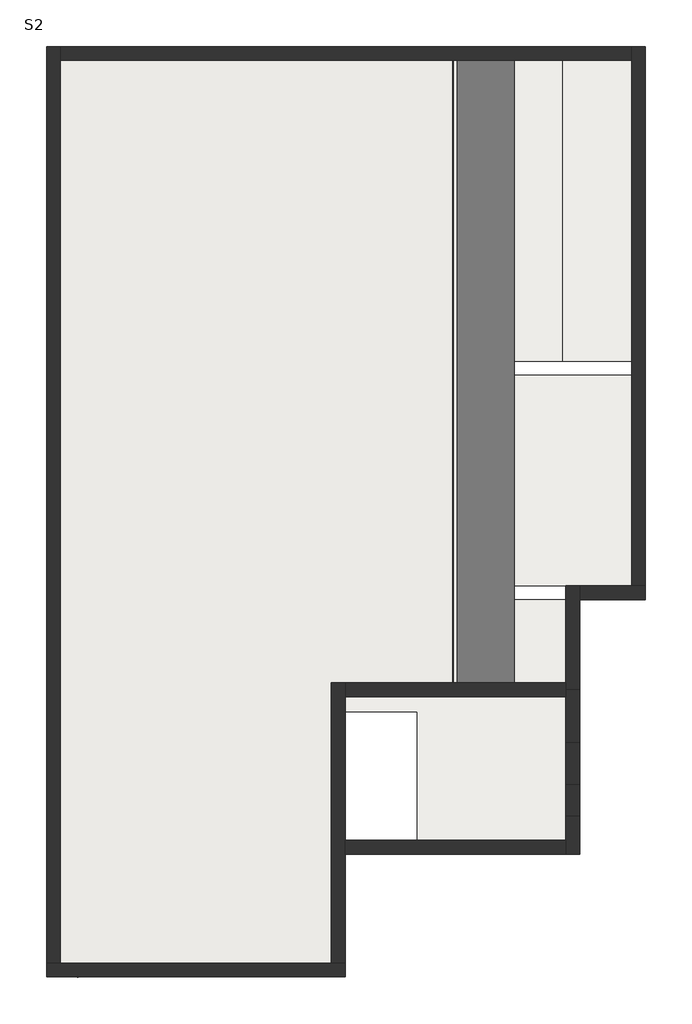
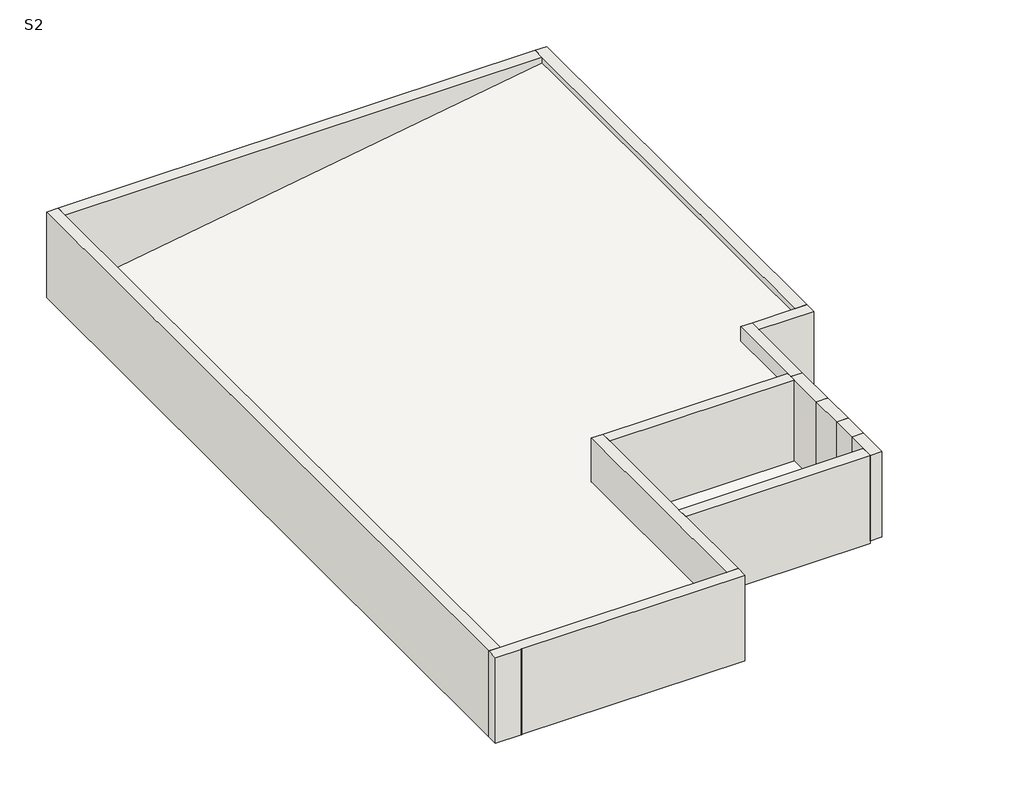
# One storey: 13 walls, 9 coverings, 2 roofs, 1 proxy.
"""IFC4 building model written with IfcOpenShell, lengths in millimetres."""

from ifc_helpers import new_model, si_unit, point, frame, frame_2d, origin, place, context, project, spatial, polyline, circle_curve, trimmed, segment, composite_curve, outline, extrude, faceted_brep, element, save
from ifc_brep_helpers import plane_surface, revolved_surface, advanced_brep

model = new_model("IFC4")

# Units and contexts
model_context = context("Model", 3, world=origin())
ifc_project = project(units=[si_unit("LENGTHUNIT", "METRE", prefix="MILLI")], contexts=[model_context])

# Site, building, storey
site = spatial("IfcSite", under=ifc_project)
building = spatial("IfcBuilding", under=site)
storey = spatial("IfcBuildingStorey", under=building, Name="S2", Elevation=7200.0)

# Proxy
placement = place(None, origin())
element("IfcBuildingElementProxy", 1, Name="Reveal", ObjectType="Reveal", at=placement, inside=storey, context=model_context, shape_type="SweptSolid", body=[
    extrude(outline(composite_curve([segment(trimmed(circle_curve(frame_2d((-9788.8712297, -10317.0014262)), 7.5), [point((-9788.8712297, -10324.5014262))], [point((-9788.8712297, -10309.5014262))], False, "CARTESIAN"), True, "CONTINUOUS"), segment(trimmed(circle_curve(frame_2d((-9788.8712297, -10317.0014262)), 7.5), [point((-9788.8712297, -10309.5014262))], [point((-9788.8712297, -10324.5014262))], False, "CARTESIAN"), True, "CONTINUOUS")], self_intersect=False)), frame((0.0, 0.0, 7200.0), z_axis=(0.0, 0.0, 1.0), x_axis=(1.0, 0.0, 0.0)), (0.0, 0.0, 1.0), 1800.0),
])

# Coverings
element("IfcCovering", 2, ObjectType="600 x 1200mm grid", at=placement, inside=storey, context=model_context, shape_type="Brep", body=[
    faceted_brep([(-8268.1448516, -9277.0014262, 6953.3191854), (-9078.1448516, -10087.0014262, 7253.3191854), (-5941.5057893, -10087.0014262, 7253.3191854), (-6751.5057893, -9277.0014262, 6953.3191854), (-8268.1448516, -9277.0014262, 6900.0), (-6751.5057893, -9277.0014262, 6900.0), (-5941.5057893, -10087.0014262, 7200.0), (-9078.1448516, -10087.0014262, 7200.0)], [[[0, 1, 2, 3]], [[4, 5, 6, 7]], [[1, 0, 4, 7]], [[2, 1, 7, 6]], [[3, 2, 6, 5]], [[0, 3, 5, 4]]]),
])
element("IfcCovering", 3, ObjectType="600 x 1200mm grid", at=placement, inside=storey, context=model_context, shape_type="SweptSolid", body=[
    extrude(outline(polyline([(-5578.8712297, -2725.4326238), (-7378.8712297, -2725.4326238), (-7378.8712297, -2955.4326238), (-5578.8712297, -2955.4326238), (-5578.8712297, -10124.3668665), (-6656.23667, -9047.0014262), (-8363.4139709, -9047.0014262), (-9403.4139709, -10087.0014262), (-10078.8712297, -10087.0014262), (-10078.8712297, -2955.4326238), (-9478.8712297, -2955.4326238), (-9478.8712297, -2725.4326238), (-10078.8712297, -2725.4326238), (-10078.8712297, -317.0014262), (-5578.8712297, -317.0014262), (-5578.8712297, -2725.4326238)])), frame((0.0, 0.0, 7150.0), z_axis=(0.0, 0.0, 1.0), x_axis=(1.0, 0.0, 0.0)), (0.0, 0.0, 1.0), 50.0),
])
element("IfcCovering", 4, ObjectType="600 x 1200mm grid", at=placement, inside=storey, context=model_context, shape_type="SweptSolid", body=[
    extrude(outline(polyline([(-5348.8712297, -5662.0014262), (-1678.8712297, -5662.0014262), (-1678.8712297, -6422.0014262), (-1678.8712297, -7122.0014262), (-1678.8712297, -7637.0014262), (-1678.8712297, -8047.0014262), (-4148.8712297, -8047.0014262), (-4148.8712297, -5912.0014262), (-5348.8712297, -5912.0014262), (-5348.8712297, -5662.0014262)])), frame((0.0, 0.0, 7150.0), z_axis=(0.0, 0.0, 1.0), x_axis=(1.0, 0.0, 0.0)), (0.0, 0.0, 1.0), 50.0),
])
element("IfcCovering", 5, ObjectType="600 x 1200mm grid", at=placement, inside=storey, context=model_context, shape_type="SweptSolid", body=[
    extrude(outline(polyline([(-5348.8712297, -5432.0014262), (-5348.8712297, -4047.0014262), (-1678.8712297, -4047.0014262), (-1678.8712297, -5432.0014262), (-5348.8712297, -5432.0014262)])), frame((0.0, 0.0, 7150.0), z_axis=(0.0, 0.0, 1.0), x_axis=(1.0, 0.0, 0.0)), (0.0, 0.0, 1.0), 50.0),
])
element("IfcCovering", 6, ObjectType="600 x 1200mm grid", at=placement, inside=storey, context=model_context, shape_type="SweptSolid", body=[
    extrude(outline(polyline([(-5348.8712297, -317.0014262), (-588.8712297, -317.0014262), (-588.8712297, -3817.0014262), (-5348.8712297, -3817.0014262), (-5348.8712297, -317.0014262)])), frame((0.0, 0.0, 7150.0), z_axis=(0.0, 0.0, 1.0), x_axis=(1.0, 0.0, 0.0)), (0.0, 0.0, 1.0), 50.0),
])
element("IfcCovering", 7, ObjectType="600 x 1200mm grid", at=placement, inside=storey, context=model_context, shape_type="SweptSolid", body=[
    extrude(outline(polyline([(-10078.8712297, 4912.9985738), (-5348.8712297, 4912.9985738), (-5348.8712297, 1822.9985738), (-5118.8712297, 1822.9985738), (-5118.8712297, 4912.9985738), (-1741.8392368, 4912.9985738), (-1741.8392368, -87.0014262), (-5118.8712297, -87.0014262), (-5118.8712297, -502.0014262), (-5348.8712297, -502.0014262), (-5348.8712297, -87.0014262), (-10078.8712297, -87.0014262), (-10078.8712297, 4912.9985738)])), frame((0.0, 0.0, 7150.0), z_axis=(0.0, 0.0, 1.0), x_axis=(1.0, 0.0, 0.0)), (0.0, 0.0, 1.0), 50.0),
])
element("IfcCovering", 8, ObjectType="600 x 1200mm grid", at=placement, inside=storey, context=model_context, shape_type="SweptSolid", body=[
    extrude(outline(polyline([(-3590.0839081, 4912.9985738), (-588.8712297, 4912.9985738), (-588.8712297, -87.0014262), (-3590.0839081, -87.0014262), (-3590.0839081, 4912.9985738)])), frame((0.0, 0.0, 7150.0), z_axis=(0.0, 0.0, 1.0), x_axis=(1.0, 0.0, 0.0)), (0.0, 0.0, 1.0), 50.0),
])
element("IfcCovering", 9, ObjectType="600 x 1200mm grid", at=placement, inside=storey, context=model_context, shape_type="SweptSolid", body=[
    extrude(outline(polyline([(-5348.8712297, -5662.0014262), (-1678.8712297, -5662.0014262), (-1678.8712297, -6422.0014262), (-1678.8712297, -7122.0014262), (-1678.8712297, -7637.0014262), (-1678.8712297, -8047.0014262), (-4148.8712297, -8047.0014262), (-4148.8712297, -5912.0014262), (-5348.8712297, -5912.0014262), (-5348.8712297, -5662.0014262)])), frame((0.0, 0.0, 7200.0), z_axis=(0.0, 0.0, 1.0), x_axis=(1.0, 0.0, 0.0)), (0.0, 0.0, 1.0), 50.0),
])
element("IfcCovering", 10, ObjectType="600 x 1200mm grid", at=placement, inside=storey, context=model_context, shape_type="SweptSolid", body=[
    extrude(outline(polyline([(-5348.8712297, -5662.0014262), (-1678.8712297, -5662.0014262), (-1678.8712297, -6422.0014262), (-1678.8712297, -7122.0014262), (-1678.8712297, -7637.0014262), (-1678.8712297, -8047.0014262), (-4148.8712297, -8047.0014262), (-4148.8712297, -5912.0014262), (-5348.8712297, -5912.0014262), (-5348.8712297, -5662.0014262)])), frame((0.0, 0.0, 7250.0), z_axis=(0.0, 0.0, 1.0), x_axis=(1.0, 0.0, 0.0)), (0.0, 0.0, 1.0), 50.0),
])

# Roofs
element("IfcRoof", 11, ObjectType="150", at=placement, inside=storey, context=model_context, shape_type="Brep", body=[
    faceted_brep([(-588.8712297, 4912.9985738, 8710.1679794), (-588.8712297, -3817.0014262, 8710.1679794), (-1678.8712297, -3817.0014262, 8536.7134907), (-1678.8712297, -5432.0014262, 8536.7134907), (-5578.8712297, -5432.0014262, 7916.0965129), (-5578.8712297, -10087.0014262, 7916.0965129), (-10078.8712297, -10087.0014262, 7200.0), (-10078.8712297, 4912.9985738, 7200.0), (-588.8712297, -3817.0014262, 8862.0553434), (-588.8712297, 4912.9985738, 8862.0553434), (-10078.8712297, 4912.9985738, 7351.887364), (-10078.8712297, -10087.0014262, 7351.887364), (-5578.8712297, -10087.0014262, 8067.9838769), (-5578.8712297, -5432.0014262, 8067.9838769), (-1678.8712297, -5432.0014262, 8688.6008548), (-1678.8712297, -3817.0014262, 8688.6008548)], [[[0, 1, 2, 3, 4, 5, 6, 7]], [[8, 9, 10, 11, 12, 13, 14, 15]], [[6, 11, 10, 7]], [[9, 8, 1, 0]], [[8, 15, 2, 1]], [[15, 14, 3, 2]], [[14, 13, 4, 3]], [[13, 12, 5, 4]], [[10, 9, 0, 7]], [[12, 11, 6, 5]]]),
])
element("IfcRoof", 12, ObjectType="2", at=placement, inside=storey, context=model_context, shape_type="Brep", body=[
    faceted_brep([(-588.8712297, 4912.9985738, 8872.0553434), (-588.8712297, -3817.0014262, 8872.0553434), (-1678.8712297, -3817.0014262, 8698.6008548), (-1678.8712297, -5432.0014262, 8698.6008548), (-5578.8712297, -5432.0014262, 8077.9838769), (-5578.8712297, -10087.0014262, 8077.9838769), (-10078.8712297, -10087.0014262, 7361.887364), (-10078.8712297, 4912.9985738, 7361.887364), (-588.8712297, -3817.0014262, 8874.0805083), (-588.8712297, 4912.9985738, 8874.0805083), (-10078.8712297, 4912.9985738, 7363.9125289), (-10078.8712297, -10087.0014262, 7363.9125289), (-5578.8712297, -10087.0014262, 8080.0090418), (-5578.8712297, -5432.0014262, 8080.0090418), (-1678.8712297, -5432.0014262, 8700.6260196), (-1678.8712297, -3817.0014262, 8700.6260196)], [[[0, 1, 2, 3, 4, 5, 6, 7]], [[8, 9, 10, 11, 12, 13, 14, 15]], [[6, 11, 10, 7]], [[9, 8, 1, 0]], [[8, 15, 2, 1]], [[15, 14, 3, 2]], [[14, 13, 4, 3]], [[13, 12, 5, 4]], [[10, 9, 0, 7]], [[12, 11, 6, 5]]]),
])

# Walls
element("IfcWall", 13, ObjectType="230", at=placement, inside=storey, context=model_context, shape_type="AdvancedBrep", body=[
    advanced_brep(
    [(-5348.8712297, -10087.0014262, 7200.0), (-5578.8712297, -10087.0014262, 7200.0), (-10078.8712297, -10087.0014262, 7200.0), (-10308.8712297, -10087.0014262, 7200.0), (-10308.8712297, -10087.0014262, 9000.0), (-10078.8712297, -10087.0014262, 9000.0), (-5578.8712297, -10087.0014262, 9000.0), (-5348.8712297, -10087.0014262, 9000.0), (-10308.8712297, -10317.0014262, 9000.0), (-10308.8712297, -10317.0014262, 7200.0), (-9796.3712297, -10317.0014262, 7200.0), (-9796.3712297, -10317.0014262, 9000.0), (-5348.8712297, -10317.0014262, 7200.0), (-5348.8712297, -10317.0014262, 9000.0), (-9781.3712297, -10317.0014262, 9000.0), (-9781.3712297, -10317.0014262, 7200.0), (-9788.8712297, -10309.5014262, 7200.0), (-9788.8712297, -10309.5014262, 9000.0)],
    [
        (0, 1),
        (1, 2),
        (2, 3),
        (3, 4),
        (4, 5),
        (5, 6),
        (6, 7),
        (7, 0),
        (8, 9),
        (9, 10),
        (10, 11),
        (11, 8),
        (12, 13),
        (13, 14),
        (14, 15),
        (15, 12),
        (0, 12),
        (15, 16, circle_curve(frame((-9788.8712297, -10317.0014262, 7200.0), z_axis=(0.0, 0.0, 1.0), x_axis=(0.0, 1.0, 0.0)), 7.5)),
        (16, 10, circle_curve(frame((-9788.8712297, -10317.0014262, 7200.0), z_axis=(0.0, 0.0, 1.0), x_axis=(0.0, 1.0, 0.0)), 7.5)),
        (9, 3),
        (4, 8),
        (11, 17, circle_curve(frame((-9788.8712297, -10317.0014262, 9000.0), z_axis=(0.0, 0.0, -1.0), x_axis=(0.0, 1.0, 0.0)), 7.5)),
        (17, 14, circle_curve(frame((-9788.8712297, -10317.0014262, 9000.0), z_axis=(0.0, 0.0, -1.0), x_axis=(0.0, 1.0, 0.0)), 7.5)),
        (13, 7),
        (16, 17),
    ],
    [
        plane_surface(frame((-5463.8712297, -10087.0014262, 7200.0), z_axis=(0.0, 1.0, 0.0), x_axis=(-1.0, 0.0, 0.0))),
        plane_surface(frame((-5463.8712297, -10317.0014262, 7200.0), z_axis=(0.0, -1.0, 0.0), x_axis=(1.0, 0.0, 0.0))),
        plane_surface(frame((-5463.8712297, -10087.0014262, 7200.0), z_axis=(0.0, 0.0, -1.0), x_axis=(0.0, -1.0, 0.0))),
        plane_surface(frame((-10193.8712297, -10087.0014262, 9000.0), z_axis=(0.0, 0.0, 1.0), x_axis=(0.0, -1.0, 0.0))),
        plane_surface(frame((-10308.8712297, -10202.0014262, 7200.0), z_axis=(-1.0, 0.0, 0.0), x_axis=(0.0, -1.0, 0.0))),
        plane_surface(frame((-5348.8712297, -10202.0014262, 7200.0), z_axis=(1.0, 0.0, 0.0), x_axis=(0.0, 1.0, 0.0))),
        revolved_surface(polyline([(-9788.8712297, -10309.5014262, 7200.0), (-9788.8712297, -10309.5014262, 9000.0)]), (-9788.8712297, -10317.0014262, 7200.0), (0.0, 0.0, -1.0)),
    ],
    [
        (0, [[1, 2, 3, 4, 5, 6, 7, 8]]),
        (1, [[9, 10, 11, 12]]),
        (1, [[13, 14, 15, 16]]),
        (2, [[-3, -2, -1, 17, -16, 18, 19, -10, 20]]),
        (3, [[-7, -6, -5, 21, -12, 22, 23, -14, 24]]),
        (4, [[-4, -20, -9, -21]]),
        (5, [[-8, -24, -13, -17]]),
        (6, [[25, -22, -11, -19]]),
        (6, [[-25, -18, -15, -23]]),
    ],
),
])
element("IfcWall", 14, ObjectType="230", at=placement, inside=storey, context=model_context, shape_type="Brep", body=[
    faceted_brep([(-10078.8712297, -10087.0014262, 7200.0), (-10078.8712297, 4912.9985738, 7200.0), (-10078.8712297, 5142.9985738, 7200.0), (-10078.8712297, 5142.9985738, 9000.0), (-10078.8712297, 4912.9985738, 9000.0), (-10078.8712297, -10087.0014262, 9000.0), (-10308.8712297, -10087.0014262, 7200.0), (-10308.8712297, -10087.0014262, 9000.0), (-10308.8712297, 5142.9985738, 9000.0), (-10308.8712297, 5142.9985738, 7200.0)], [[[0, 1, 2, 3, 4, 5]], [[6, 7, 8, 9]], [[2, 1, 0, 6, 9]], [[5, 4, 3, 8, 7]], [[0, 5, 7, 6]], [[3, 2, 9, 8]]]),
])
element("IfcWall", 15, ObjectType="230", at=placement, inside=storey, context=model_context, shape_type="Brep", body=[
    faceted_brep([(-5348.8712297, -10087.0014262, 7200.0), (-5348.8712297, -5662.0014262, 7200.0), (-5348.8712297, -5432.0014262, 7200.0), (-5348.8712297, -5432.0014262, 9000.0), (-5348.8712297, -5662.0014262, 9000.0), (-5348.8712297, -8047.0014262, 9000.0), (-5348.8712297, -8277.0014262, 9000.0), (-5348.8712297, -10087.0014262, 9000.0), (-5578.8712297, -10087.0014262, 7200.0), (-5578.8712297, -10087.0014262, 9000.0), (-5578.8712297, -5432.0014262, 9000.0), (-5578.8712297, -5432.0014262, 7200.0)], [[[0, 1, 2, 3, 4, 5, 6, 7]], [[8, 9, 10, 11]], [[2, 1, 0, 8, 11]], [[7, 6, 5, 4, 3, 10, 9]], [[0, 7, 9, 8]], [[3, 2, 11, 10]]]),
])
element("IfcWall", 16, ObjectType="230", at=placement, inside=storey, context=model_context, shape_type="Brep", body=[
    faceted_brep([(-5348.8712297, -8277.0014262, 7150.0), (-1678.8712297, -8277.0014262, 7150.0), (-1678.8712297, -8277.0014262, 7200.0), (-1678.8712297, -8277.0014262, 9000.0), (-5348.8712297, -8277.0014262, 9000.0), (-5348.8712297, -8047.0014262, 7150.0), (-5348.8712297, -8047.0014262, 9000.0), (-1678.8712297, -8047.0014262, 9000.0), (-1678.8712297, -8047.0014262, 7150.0)], [[[0, 1, 2, 3, 4]], [[5, 6, 7, 8]], [[1, 0, 5, 8]], [[4, 3, 7, 6]], [[0, 4, 6, 5]], [[3, 2, 1, 8, 7]]]),
])
element("IfcWall", 17, ObjectType="230", at=placement, inside=storey, context=model_context, shape_type="Brep", body=[
    faceted_brep([(-1678.8712297, -5547.0014262, 7150.0), (-1678.8712297, -6422.0014262, 7150.0), (-1678.8712297, -6422.0014262, 7200.0), (-1678.8712297, -6422.0014262, 9000.0), (-1678.8712297, -5662.0014262, 9000.0), (-1678.8712297, -5547.0014262, 9000.0), (-1678.8712297, -5547.0014262, 7200.0), (-1448.8712297, -5547.0014262, 7150.0), (-1448.8712297, -5547.0014262, 7200.0), (-1448.8712297, -5547.0014262, 9000.0), (-1448.8712297, -6422.0014262, 9000.0), (-1448.8712297, -6422.0014262, 7200.0), (-1448.8712297, -6422.0014262, 7150.0)], [[[0, 1, 2, 3, 4, 5, 6]], [[7, 8, 9, 10, 11, 12]], [[1, 0, 7, 12]], [[3, 2, 1, 12, 11, 10]], [[5, 4, 3, 10, 9]], [[0, 6, 5, 9, 8, 7]]]),
])
element("IfcWall", 18, ObjectType="230", at=placement, inside=storey, context=model_context, shape_type="Brep", body=[
    faceted_brep([(-1678.8712297, -7122.0014262, 7150.0), (-1678.8712297, -7637.0014262, 7150.0), (-1678.8712297, -7637.0014262, 7200.0), (-1678.8712297, -7637.0014262, 9000.0), (-1678.8712297, -7122.0014262, 9000.0), (-1678.8712297, -7122.0014262, 7200.0), (-1448.8712297, -7122.0014262, 7150.0), (-1448.8712297, -7122.0014262, 7200.0), (-1448.8712297, -7122.0014262, 9000.0), (-1448.8712297, -7637.0014262, 9000.0), (-1448.8712297, -7637.0014262, 7200.0), (-1448.8712297, -7637.0014262, 7150.0)], [[[0, 1, 2, 3, 4, 5]], [[6, 7, 8, 9, 10, 11]], [[1, 0, 6, 11]], [[3, 2, 1, 11, 10, 9]], [[4, 3, 9, 8]], [[0, 5, 4, 8, 7, 6]]]),
])
element("IfcWall", 19, ObjectType="230", at=placement, inside=storey, context=model_context, shape_type="SweptSolid", body=[
    extrude(outline(polyline([(-1678.8712297, -7122.0014262), (-1678.8712297, -6422.0014262), (-1448.8712297, -6422.0014262), (-1448.8712297, -7122.0014262), (-1678.8712297, -7122.0014262)])), frame((0.0, 0.0, 7200.0), z_axis=(0.0, 0.0, 1.0), x_axis=(1.0, 0.0, 0.0)), (0.0, 0.0, 1.0), 1800.0),
])
element("IfcWall", 20, ObjectType="230", at=placement, inside=storey, context=model_context, shape_type="Brep", body=[
    faceted_brep([(-1678.8712297, -7637.0014262, 7200.0), (-1678.8712297, -8277.0014262, 7200.0), (-1678.8712297, -8277.0014262, 9000.0), (-1678.8712297, -8047.0014262, 9000.0), (-1678.8712297, -7637.0014262, 9000.0), (-1448.8712297, -7637.0014262, 7200.0), (-1448.8712297, -7637.0014262, 9000.0), (-1448.8712297, -8277.0014262, 9000.0), (-1448.8712297, -8277.0014262, 7200.0)], [[[0, 1, 2, 3, 4]], [[5, 6, 7, 8]], [[1, 0, 5, 8]], [[4, 3, 2, 7, 6]], [[0, 4, 6, 5]], [[2, 1, 8, 7]]]),
])
element("IfcWall", 21, ObjectType="230", at=placement, inside=storey, context=model_context, shape_type="Brep", body=[
    faceted_brep([(-1448.8712297, -5547.0014262, 7200.0), (-1448.8712297, -4047.0014262, 7200.0), (-1448.8712297, -3817.0014262, 7200.0), (-1448.8712297, -3817.0014262, 9000.0), (-1448.8712297, -4047.0014262, 9000.0), (-1448.8712297, -5547.0014262, 9000.0), (-1678.8712297, -5547.0014262, 7200.0), (-1678.8712297, -5547.0014262, 9000.0), (-1678.8712297, -5432.0014262, 9000.0), (-1678.8712297, -3817.0014262, 9000.0), (-1678.8712297, -3817.0014262, 7200.0), (-1678.8712297, -5432.0014262, 7200.0)], [[[0, 1, 2, 3, 4, 5]], [[6, 7, 8, 9, 10, 11]], [[2, 1, 0, 6, 11, 10]], [[5, 4, 3, 9, 8, 7]], [[0, 5, 7, 6]], [[3, 2, 10, 9]]]),
])
element("IfcWall", 22, ObjectType="230", at=placement, inside=storey, context=model_context, shape_type="Brep", body=[
    faceted_brep([(-1448.8712297, -4047.0014262, 7200.0), (-358.8712297, -4047.0014262, 7200.0), (-358.8712297, -4047.0014262, 9000.0), (-1448.8712297, -4047.0014262, 9000.0), (-1448.8712297, -3817.0014262, 7200.0), (-1448.8712297, -3817.0014262, 9000.0), (-588.8712297, -3817.0014262, 9000.0), (-358.8712297, -3817.0014262, 9000.0), (-358.8712297, -3817.0014262, 7200.0), (-588.8712297, -3817.0014262, 7200.0)], [[[0, 1, 2, 3]], [[4, 5, 6, 7, 8, 9]], [[1, 0, 4, 9, 8]], [[3, 2, 7, 6, 5]], [[0, 3, 5, 4]], [[2, 1, 8, 7]]]),
])
element("IfcWall", 23, ObjectType="230", at=placement, inside=storey, context=model_context, shape_type="Brep", body=[
    faceted_brep([(-358.8712297, -3817.0014262, 7200.0), (-358.8712297, 5142.9985738, 7200.0), (-358.8712297, 5142.9985738, 9000.0), (-358.8712297, -3817.0014262, 9000.0), (-588.8712297, -3817.0014262, 7200.0), (-588.8712297, -3817.0014262, 9000.0), (-588.8712297, 4912.9985738, 9000.0), (-588.8712297, 5142.9985738, 9000.0), (-588.8712297, 5142.9985738, 7200.0), (-588.8712297, 4912.9985738, 7200.0)], [[[0, 1, 2, 3]], [[4, 5, 6, 7, 8, 9]], [[1, 0, 4, 9, 8]], [[3, 2, 7, 6, 5]], [[0, 3, 5, 4]], [[2, 1, 8, 7]]]),
])
element("IfcWall", 24, ObjectType="230", at=placement, inside=storey, context=model_context, shape_type="SweptSolid", body=[
    extrude(outline(polyline([(-588.8712297, 4912.9985738), (-10078.8712297, 4912.9985738), (-10078.8712297, 5142.9985738), (-588.8712297, 5142.9985738), (-588.8712297, 4912.9985738)])), frame((0.0, 0.0, 7200.0), z_axis=(0.0, 0.0, 1.0), x_axis=(1.0, 0.0, 0.0)), (0.0, 0.0, 1.0), 1800.0),
])
element("IfcWall", 25, ObjectType="230", at=placement, inside=storey, context=model_context, shape_type="Brep", body=[
    faceted_brep([(-5348.8712297, -5662.0014262, 7200.0), (-1678.8712297, -5662.0014262, 7200.0), (-1678.8712297, -5662.0014262, 9000.0), (-5348.8712297, -5662.0014262, 9000.0), (-5348.8712297, -5432.0014262, 7200.0), (-5348.8712297, -5432.0014262, 9000.0), (-1678.8712297, -5432.0014262, 9000.0), (-1678.8712297, -5432.0014262, 7200.0), (-1678.8712297, -5547.0014262, 7200.0), (-1678.8712297, -5547.0014262, 9000.0)], [[[0, 1, 2, 3]], [[4, 5, 6, 7]], [[1, 0, 4, 7, 8]], [[3, 2, 9, 6, 5]], [[2, 1, 8, 7, 6, 9]], [[0, 3, 5, 4]]]),
])

save(model, "model.ifc")

# Revit data of these elements
# Type "600 x 1200mm grid"
#   built-in parameter 1002203 = 1 (stored number, unit not read)
#   built-in parameter 1002202 = 1 (stored number, unit not read)
#   Layers, outside or top first: 25 mm "J POP CEILING" (function 1); 25 mm "J POP CEILING" (function 5)
# Type "150"
#   Layers, outside or top first: 150 mm "J ROOF" (function 1)
# Type "2"
#   Layers, outside or top first: 2 mm "J ROOF 2" (function 1)
# Type "230"
#   Layers, outside or top first: 230 mm "Default Wall" (function 1)
# Element 2 (IfcCovering, "600 x 1200mm grid")
#   Height Offset From Level = -300 mm
#   Phase Created = New Construction
#   Materials on its faces: "J POP CEILING"
# Elements 3, 4, 5, 6, 7, 8 (IfcCovering, "600 x 1200mm grid")
#   Height Offset From Level = -50 mm
#   Phase Created = New Construction
#   Materials on its faces: "J POP CEILING"
# Element 9 (IfcCovering, "600 x 1200mm grid")
#   Height Offset From Level = 0 mm
#   Phase Created = New Construction
#   Materials on its faces: "J POP CEILING"
# Element 10 (IfcCovering, "600 x 1200mm grid")
#   Height Offset From Level = 50 mm
#   Phase Created = New Construction
#   Materials on its faces: "J POP CEILING"
# Element 11 (IfcRoof, "150")
#   built-in parameter 1001705 = 29.075 (stored number, unit not read)
#   built-in parameter 1001710 = 33615
#   Phase Created = New Construction
#   Materials on its faces: "J ROOF"
# Element 12 (IfcRoof, "2")
#   built-in parameter 1001705 = 29.1144 (stored number, unit not read)
#   built-in parameter 1001701 = 0.531127 (stored number, unit not read)
#   built-in parameter 1001710 = 33615
#   Phase Created = New Construction
#   Materials on its faces: "J ROOF 2"
# Elements 13, 14, 15, 19, 20, 21, 22, 23, 24, 25 (IfcWall, "230")
#   Top Offset = -1650 mm
#   Base Offset = 0 mm
#   wall height = 1800 mm
#   Phase Created = New Construction
#   Base Constraint = S2
#   Top Constraint = 04-ROOF PLAN
#   Materials on its faces: "Default Wall"
# Elements 16, 17, 18 (IfcWall, "230")
#   built-in parameter 1001111 = -50 mm
#   Top Offset = -1650 mm
#   Base Offset = -50 mm
#   wall height = 1850 mm
#   Phase Created = New Construction
#   Base Constraint = S2
#   Top Constraint = 04-ROOF PLAN
#   Materials on its faces: "Default Wall"
# Materials
#   "J POP CEILING": class "Generic", colour RGB 255 255 255, transparency 0, Cost = 0
#   "J ROOF": class "Generic", colour RGB 255 255 255, transparency 0, Cost = 0
#   "J ROOF 2": class "Generic", colour RGB 120 120 120, transparency 0, Cost = 0
#   "Default Wall": colour RGB 255 255 255, transparency 0, Cost = 0
